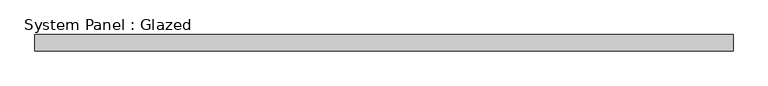
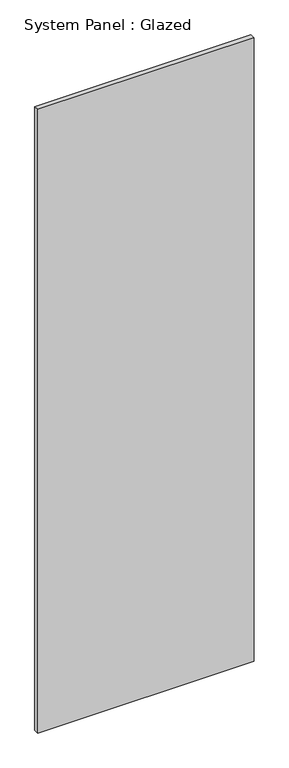
"""IFC4 building model written with IfcOpenShell, lengths in millimetres: plate geometry, System Panel : Glazed."""

from ifc_helpers import new_model, si_unit, origin, origin_with_axes, place, context, project, spatial, polyline, outline, extrude, source, transform, mapped, element, save


def system_panel_glazed_8a71b067(model_context):
    return source(origin(), model_context, "Body", "SweptSolid", [
        extrude(outline(polyline([(546.1, 19.05), (-546.1, 19.05), (-546.1, 44.45), (546.1, 44.45), (546.1, 19.05)])), origin_with_axes(), (0.0, 0.0, 1.0), 3327.000116),
    ])


if __name__ == "__main__":
    model = new_model("IFC4")
    model_context = context("Model", 3, world=origin())
    ifc_project = project(units=[si_unit("LENGTHUNIT", "METRE", prefix="MILLI")], contexts=[model_context])
    site = spatial("IfcSite", under=ifc_project)
    building = spatial("IfcBuilding", under=site)
    placement = place(None, origin())
    system_panel_glazed_shape = system_panel_glazed_8a71b067(model_context)
    element("IfcPlate", 1, ObjectType="System Panel : Glazed", at=placement, inside=building, context=model_context, shape_type="MappedRepresentation", body=[
        mapped(system_panel_glazed_shape, transform((0.0, 0.0, 0.0), x_axis=(1.0, 0.0, 0.0), y_axis=(0.0, 1.0, 0.0), z_axis=(0.0, 0.0, 1.0))),
    ])
    save(model, "model.ifc")

# Revit data of these elements
# Type "System Panel : Glazed"
#   Construction Type Id = "GSP4R"
#   Analytic Construction = "1/8 in Pilkington single glazing"
#   Visual Light Transmittance = 0.9
#   Solar Heat Gain Coefficient = 0.86
#   Heat Transfer Coefficient (U) = 1.18115 BTU/(h·ft²·°F)
#   Define Thermal Properties by = 1
# Element 1 (IfcPlate, "System Panel : Glazed")
#   Materials on its faces: "Glass"
# Materials
#   "Glass": class "Glass", colour RGB 0 128 192, transparency 0.75, Description = "Soda Lime Glass", Cost = 0
